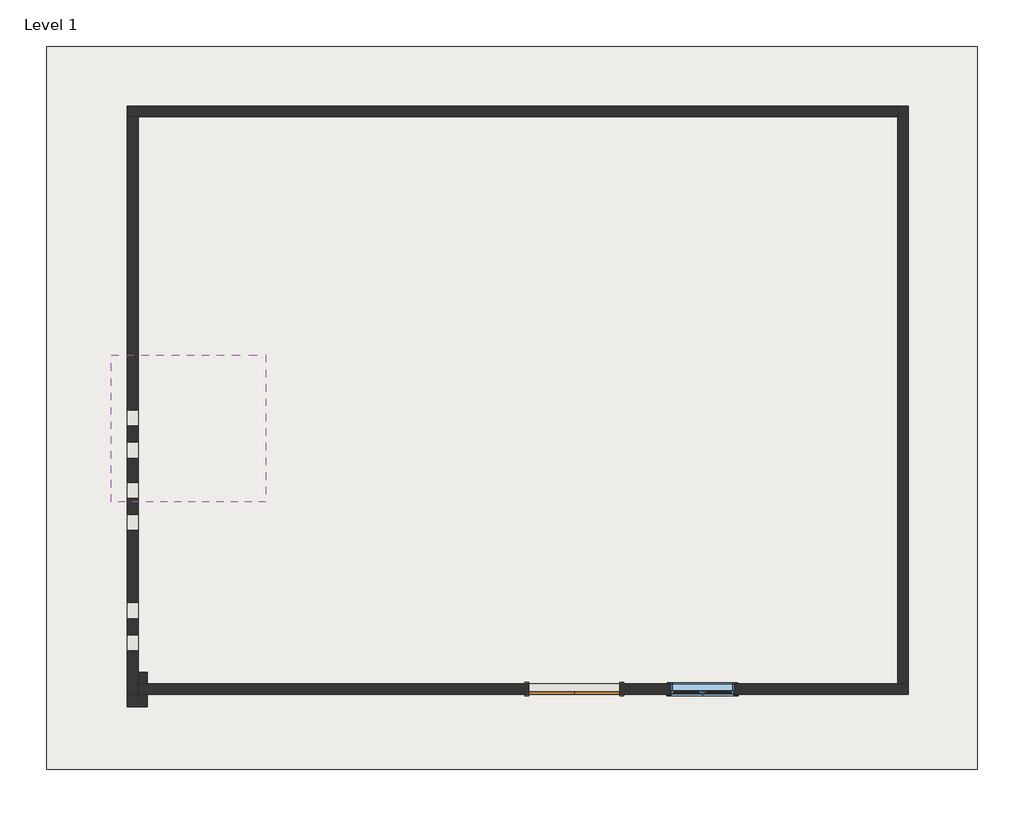
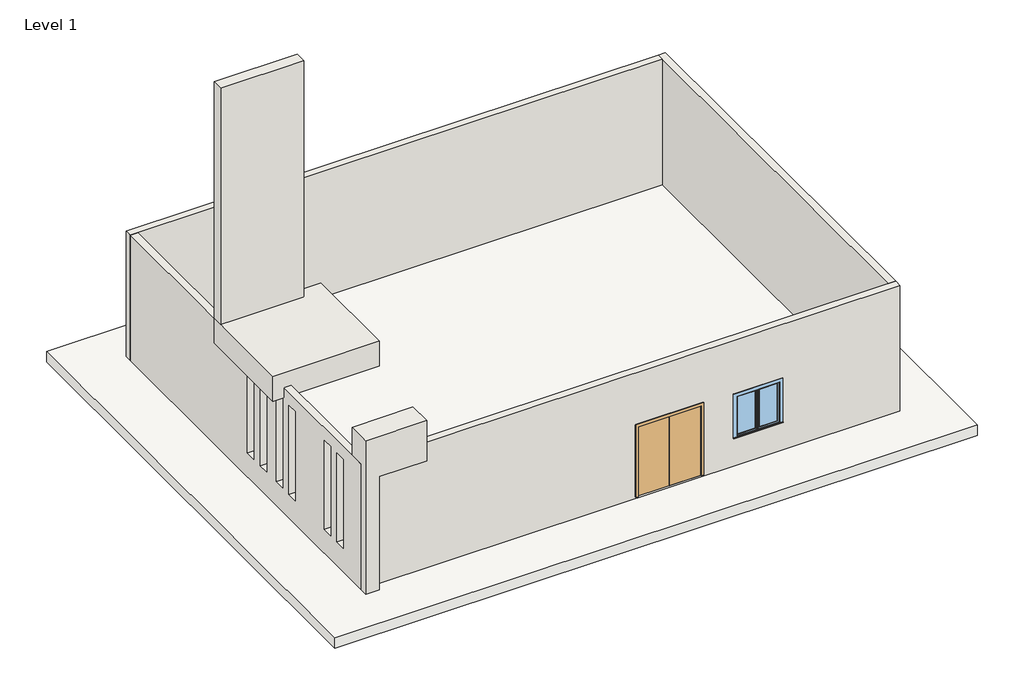
# One storey: 6 walls, 1 door, 1 slab, 1 window.
"""IFC4 building model written with IfcOpenShell, lengths in millimetres."""

from ifc_helpers import new_model, si_unit, frame, origin, place, context, project, spatial, polyline, outline, extrude, faceted_brep, transform, mapped, element, save
from components import door_aae36eb6, walls_3_walls_3_66379a57, walls_5_walls_5_4d7304d2, window_0862ab64

model = new_model("IFC4")

# Units and contexts
model_context = context("Model", 3, world=origin())
ifc_project = project(units=[si_unit("LENGTHUNIT", "METRE", prefix="MILLI")], contexts=[model_context])

# Site, building, storey
site = spatial("IfcSite", under=ifc_project)
building = spatial("IfcBuilding", under=site)
storey = spatial("IfcBuildingStorey", under=building, Name="Level 1", Elevation=0.0)

# Door
placement = place(None, origin())
door_shape = door_aae36eb6(model_context)
element("IfcDoor", 1, ObjectType="Door-Double-Flush_Panel : 68\" x 80\"", at=placement, inside=storey, context=model_context, shape_type="MappedRepresentation", body=[
    mapped(door_shape, transform((-2725.0620963, -3310.4885822, 50.8), x_axis=(-1.0, 0.0, 0.0), y_axis=(0.0, -1.0, 0.0), z_axis=(0.0, 0.0, 1.0))),
])

# Slab
element("IfcSlab", 2, ObjectType="Generic - 12\"", at=placement, inside=storey, context=model_context, shape_type="SweptSolid", body=[
    extrude(outline(polyline([(4934.5944472, 8897.8612165), (4934.5944472, -4834.4885822), (-12743.8055528, -4834.4885822), (-12743.8055528, 8897.8612165), (4934.5944472, 8897.8612165)])), frame((0.0, 0.0, -304.8), z_axis=(0.0, 0.0, 1.0), x_axis=(1.0, 0.0, 0.0)), (0.0, 0.0, 1.0), 304.8),
])

# Walls
element("IfcWall", 3, ObjectType="Generic - 8\"", at=placement, inside=storey, context=model_context, shape_type="Brep", body=[
    faceted_brep([(-11208.6620963, 7560.7114178, 0.0), (-11005.4620963, 7560.7114178, 0.0), (3421.7379037, 7560.7114178, 0.0), (3421.7379037, 7560.7114178, 3657.6), (-11005.4620963, 7560.7114178, 3657.6), (-11208.6620963, 7560.7114178, 3657.6), (-11208.6620963, 7763.9114178, 0.0), (-11208.6620963, 7763.9114178, 3657.6), (3421.7379037, 7763.9114178, 3657.6), (3421.7379037, 7763.9114178, 0.0)], [[[0, 1, 2, 3, 4, 5]], [[6, 7, 8, 9]], [[2, 1, 0, 6, 9]], [[0, 5, 7, 6]], [[3, 2, 9, 8]], [[5, 4, 3, 8, 7]]]),
])
element("IfcWall", 4, ObjectType="Generic - 8\"", at=placement, inside=storey, context=model_context, shape_type="Brep", body=[
    faceted_brep([(-11005.4620963, -3412.0885822, 0.0), (-11005.4620963, -3208.8885822, 0.0), (-11005.4620963, 7560.7114178, 0.0), (-11005.4620963, 7560.7114178, 3657.6), (-11005.4620963, -3208.8885822, 3657.6), (-11005.4620963, -3412.0885822, 3657.6), (-11005.4620963, -2583.9937304, 3288.4675072), (-11005.4620963, -2279.1937304, 3288.4675072), (-11005.4620963, -2279.1937304, 697.6675072), (-11005.4620963, -2583.9937304, 697.6675072), (-11005.4620963, -1974.3937304, 3288.4675072), (-11005.4620963, -1669.5937304, 3288.4675072), (-11005.4620963, -1669.5937304, 697.6675072), (-11005.4620963, -1974.3937304, 697.6675072), (-11005.4620963, -297.9937304, 3288.4675072), (-11005.4620963, 6.8062696, 3288.4675072), (-11005.4620963, 6.8062696, 697.6675072), (-11005.4620963, -297.9937304, 697.6675072), (-11005.4620963, 311.6062696, 3288.4675072), (-11005.4620963, 616.4062696, 3288.4675072), (-11005.4620963, 616.4062696, 697.6675072), (-11005.4620963, 311.6062696, 697.6675072), (-11005.4620963, 1073.6062696, 3288.4675072), (-11005.4620963, 1378.4062696, 3288.4675072), (-11005.4620963, 1378.4062696, 697.6675072), (-11005.4620963, 1073.6062696, 697.6675072), (-11005.4620963, 1683.2062696, 3288.4675072), (-11005.4620963, 1988.0062696, 3288.4675072), (-11005.4620963, 1988.0062696, 697.6675072), (-11005.4620963, 1683.2062696, 697.6675072), (-11208.6620963, -3412.0885822, 0.0), (-11208.6620963, -3412.0885822, 3657.6), (-11208.6620963, 7560.7114178, 3657.6), (-11208.6620963, 7560.7114178, 0.0), (-11208.6620963, -2583.9937304, 3288.4675072), (-11208.6620963, -2583.9937304, 697.6675072), (-11208.6620963, -2279.1937304, 697.6675072), (-11208.6620963, -2279.1937304, 3288.4675072), (-11208.6620963, -1974.3937304, 3288.4675072), (-11208.6620963, -1974.3937304, 697.6675072), (-11208.6620963, -1669.5937304, 697.6675072), (-11208.6620963, -1669.5937304, 3288.4675072), (-11208.6620963, -297.9937304, 3288.4675072), (-11208.6620963, -297.9937304, 697.6675072), (-11208.6620963, 6.8062696, 697.6675072), (-11208.6620963, 6.8062696, 3288.4675072), (-11208.6620963, 311.6062696, 3288.4675072), (-11208.6620963, 311.6062696, 697.6675072), (-11208.6620963, 616.4062696, 697.6675072), (-11208.6620963, 616.4062696, 3288.4675072), (-11208.6620963, 1073.6062696, 3288.4675072), (-11208.6620963, 1073.6062696, 697.6675072), (-11208.6620963, 1378.4062696, 697.6675072), (-11208.6620963, 1378.4062696, 3288.4675072), (-11208.6620963, 1683.2062696, 3288.4675072), (-11208.6620963, 1683.2062696, 697.6675072), (-11208.6620963, 1988.0062696, 697.6675072), (-11208.6620963, 1988.0062696, 3288.4675072)], [[[0, 1, 2, 3, 4, 5], [6, 7, 8, 9], [10, 11, 12, 13], [14, 15, 16, 17], [18, 19, 20, 21], [22, 23, 24, 25], [26, 27, 28, 29]], [[30, 31, 32, 33], [34, 35, 36, 37], [38, 39, 40, 41], [42, 43, 44, 45], [46, 47, 48, 49], [50, 51, 52, 53], [54, 55, 56, 57]], [[0, 5, 31, 30]], [[3, 2, 33, 32]], [[5, 4, 3, 32, 31]], [[2, 1, 0, 30, 33]], [[7, 6, 34, 37]], [[8, 7, 37, 36]], [[9, 8, 36, 35]], [[6, 9, 35, 34]], [[11, 10, 38, 41]], [[12, 11, 41, 40]], [[13, 12, 40, 39]], [[10, 13, 39, 38]], [[15, 14, 42, 45]], [[16, 15, 45, 44]], [[17, 16, 44, 43]], [[14, 17, 43, 42]], [[19, 18, 46, 49]], [[20, 19, 49, 48]], [[21, 20, 48, 47]], [[18, 21, 47, 46]], [[23, 22, 50, 53]], [[24, 23, 53, 52]], [[25, 24, 52, 51]], [[22, 25, 51, 50]], [[27, 26, 54, 57]], [[28, 27, 57, 56]], [[29, 28, 56, 55]], [[26, 29, 55, 54]]]),
])
element("IfcWall", 5, ObjectType="Generic - 8\"", at=placement, inside=storey, context=model_context, shape_type="Brep", body=[
    faceted_brep([(3624.9379037, -3208.8885822, 0.0), (3421.7379037, -3208.8885822, 0.0), (-11005.4620963, -3208.8885822, 0.0), (-11005.4620963, -3208.8885822, 3657.6), (3421.7379037, -3208.8885822, 3657.6), (3624.9379037, -3208.8885822, 3657.6), (-3588.6620963, -3208.8885822, 2082.8), (-3588.6620963, -3208.8885822, 50.8), (-1861.4620963, -3208.8885822, 50.8), (-1861.4620963, -3208.8885822, 2082.8), (-896.2620963, -3208.8885822, 2032.0), (-896.2620963, -3208.8885822, 812.8), (322.9379037, -3208.8885822, 812.8), (322.9379037, -3208.8885822, 2032.0), (-11005.4620963, -3412.0885822, 0.0), (3624.9379037, -3412.0885822, 0.0), (3624.9379037, -3412.0885822, 3657.6), (-11005.4620963, -3412.0885822, 3657.6), (-3588.6620963, -3412.0885822, 50.8), (-3588.6620963, -3412.0885822, 2082.8), (-1861.4620963, -3412.0885822, 2082.8), (-1861.4620963, -3412.0885822, 50.8), (-896.2620963, -3412.0885822, 812.8), (-896.2620963, -3412.0885822, 2032.0), (322.9379037, -3412.0885822, 2032.0), (322.9379037, -3412.0885822, 812.8)], [[[0, 1, 2, 3, 4, 5], [6, 7, 8, 9], [10, 11, 12, 13]], [[14, 15, 16, 17], [18, 19, 20, 21], [22, 23, 24, 25]], [[2, 1, 0, 15, 14]], [[0, 5, 16, 15]], [[3, 2, 14, 17]], [[5, 4, 3, 17, 16]], [[18, 7, 6, 19]], [[19, 6, 9, 20]], [[20, 9, 8, 21]], [[7, 18, 21, 8]], [[11, 10, 23, 22]], [[12, 11, 22, 25]], [[13, 12, 25, 24]], [[10, 13, 24, 23]]]),
])
element("IfcWall", 6, ObjectType="Generic - 8\"", at=placement, inside=storey, context=model_context, shape_type="Brep", body=[
    faceted_brep([(3421.7379037, 7763.9114178, 0.0), (3421.7379037, 7560.7114178, 0.0), (3421.7379037, -3208.8885822, 0.0), (3421.7379037, -3208.8885822, 3657.6), (3421.7379037, 7560.7114178, 3657.6), (3421.7379037, 7763.9114178, 3657.6), (3624.9379037, 7763.9114178, 0.0), (3624.9379037, 7763.9114178, 3657.6), (3624.9379037, -3208.8885822, 3657.6), (3624.9379037, -3208.8885822, 0.0)], [[[0, 1, 2, 3, 4, 5]], [[6, 7, 8, 9]], [[2, 1, 0, 6, 9]], [[0, 5, 7, 6]], [[3, 2, 9, 8]], [[5, 4, 3, 8, 7]]]),
])
walls_3_walls_3_shape = walls_3_walls_3_66379a57(model_context)
element("IfcWall", 7, ObjectType="Walls 3 : Walls 3", at=placement, inside=storey, context=model_context, shape_type="MappedRepresentation", body=[
    mapped(walls_3_walls_3_shape, transform((0.0, 0.0, 0.0), x_axis=(1.0, 0.0, 0.0), y_axis=(0.0, 1.0, 0.0), z_axis=(0.0, 0.0, 1.0))),
])
walls_5_walls_5_shape = walls_5_walls_5_4d7304d2(model_context)
element("IfcWall", 8, ObjectType="Walls 5 : Walls 5", at=placement, inside=storey, context=model_context, shape_type="MappedRepresentation", body=[
    mapped(walls_5_walls_5_shape, transform((0.0, 0.0, 0.0), x_axis=(1.0, 0.0, 0.0), y_axis=(0.0, 1.0, 0.0), z_axis=(0.0, 0.0, 1.0))),
])

# Window
window_shape = window_0862ab64(model_context)
element("IfcWindow", 9, ObjectType="Casement Dbl with Trim.0001 : 48\" x 48\"", at=placement, inside=storey, context=model_context, shape_type="MappedRepresentation", body=[
    mapped(window_shape, transform((-286.6620963, -3291.4385822, -101.6), x_axis=(-1.0, 0.0, 0.0), y_axis=(0.0, -1.0, 0.0), z_axis=(0.0, 0.0, 1.0))),
])

save(model, "model.ifc")

# Revit data of these elements
# Type "Door-Double-Flush_Panel : 68\" x 80\""
#   Type Mark = "8"
#   Construction Type Id = "DOOR"
#   Assembly Code = "C1020"
#   Analytic Construction = "Wooden"
#   Thickness = 0' - 2"
#   Thermal Resistance (R) = 2.5876 (h·ft²·°F)/BTU
#   Swing Angle [instance default] = 90.00°
#   Panel Width = 2' - 10"
#   Heat Transfer Coefficient (U) = 0.3865 BTU/(h·ft²·°F)
#   Height = 6' - 8"
#   Trim Projection Ext = 0' - 1"
#   Trim Projection Int = 0' - 1"
#   Trim Width = 0' - 3"
#   Width = 5' - 8"
#   Define Thermal Properties by = 1
#   Panel Material = Wood - Birch - Solid Stained Light Low Gloss
#   Trim Material = Paint - Sienna
#   Visual Light Transmittance = 0
#   Solar Heat Gain Coefficient = 0
#   Function = (empty or 0)
#   Wall Closure = (empty or 0)
# Type "Generic - 12\""
#   Assembly Code = "B1010"
#   Function = 0
#   Layers, outside or top first: 1' - 0" no material (function 1)
# Type "Generic - 8\""
#   Assembly Code = "B2010"
#   Layers, outside or top first: 0' - 8" no material (function 1)
# Type "Casement Dbl with Trim.0001 : 48\" x 48\""
#   Type Mark = "10"
#   Construction Type Id = "GSP4R"
#   Assembly Code = "B2020100"
#   Analytic Construction = "1/8 in Pilkington single glazing"
#   Visual Light Transmittance = 0.9
#   Solar Heat Gain Coefficient = 0.78
#   Heat Transfer Coefficient (U) = 0.6496 BTU/(h·ft²·°F)
#   Height = 4' - 0"
#   Default Sill Height = 3' - 0"
#   Trim Projection - Ext. = 0' - 0 1/2"
#   Trim Projection - Int. = 0' - 0 3/4"
#   Trim Width - Exterior = 0' - 3 1/2"
#   Trim Width - Interior = 0' - 3 1/2"
#   Width = 4' - 0"
#   Window Inset = 0' - 0 3/4"
#   Define Thermal Properties by = 1
#   Glass Pane Material = Glass
#   Sash Material = Sash
#   Trim Exterior Material = Trim
#   Trim Interior Material = Trim
#   Wall Closure = (empty or 0)
# Element 1 (IfcDoor, "Door-Double-Flush_Panel : 68\" x 80\"")
#   Swing Angle = 90.00°
#   Phase Created = New Construction
#   Materials on its faces: "Paint - Sienna", "Wood - Birch - Solid Stained Light Low Gloss"
# Element 2 (IfcSlab, "Generic - 12\"")
#   Height Offset From Level = 0' - 0"
#   Phase Created = New Construction
#   Materials on its faces: "Default Floor"
# Elements 3, 4, 5, 6 (IfcWall, "Generic - 8\"")
#   Top Offset = 0' - 0"
#   Base Offset = 0' - 0"
#   Unconnected Height = 12' - 0"
#   wall height = 12' - 0"
#   Phase Created = New Construction
#   Base Constraint = Level 1
#   Materials on its faces: "Default Wall"
# Element 7 (IfcWall, "Walls 3 : Walls 3")
#   Phase Created = New Construction
#   Materials on its faces: "Default Wall"
# Element 8 (IfcWall, "Walls 5 : Walls 5")
#   Phase Created = New Construction
#   Materials on its faces: "Default Wall"
# Element 9 (IfcWindow, "Casement Dbl with Trim.0001 : 48\" x 48\"")
#   Mark = "7"
#   Phase Created = New Construction
#   Materials on its faces: "Sash", "Trim", "Glass"
# Materials
#   "Wood - Birch - Solid Stained Light Low Gloss": class "Wood", colour RGB 210 159 95, transparency 0, Cost = 0
#   "Paint - Sienna": colour RGB 118 70 51, transparency 0, Cost = 0
#   "Glass": class "Glass", colour RGB 0 128 192, transparency 0.75, Description = "Soda Lime Glass", Cost = 0
#   "Sash": class "Wood", colour RGB 224 178 126, transparency 0
#   "Trim": class "Wood", colour RGB 224 178 126, transparency 0
#   "Default Floor": colour RGB 128 128 128, transparency 0
#   "Default Wall": colour RGB 128 128 128, transparency 0
